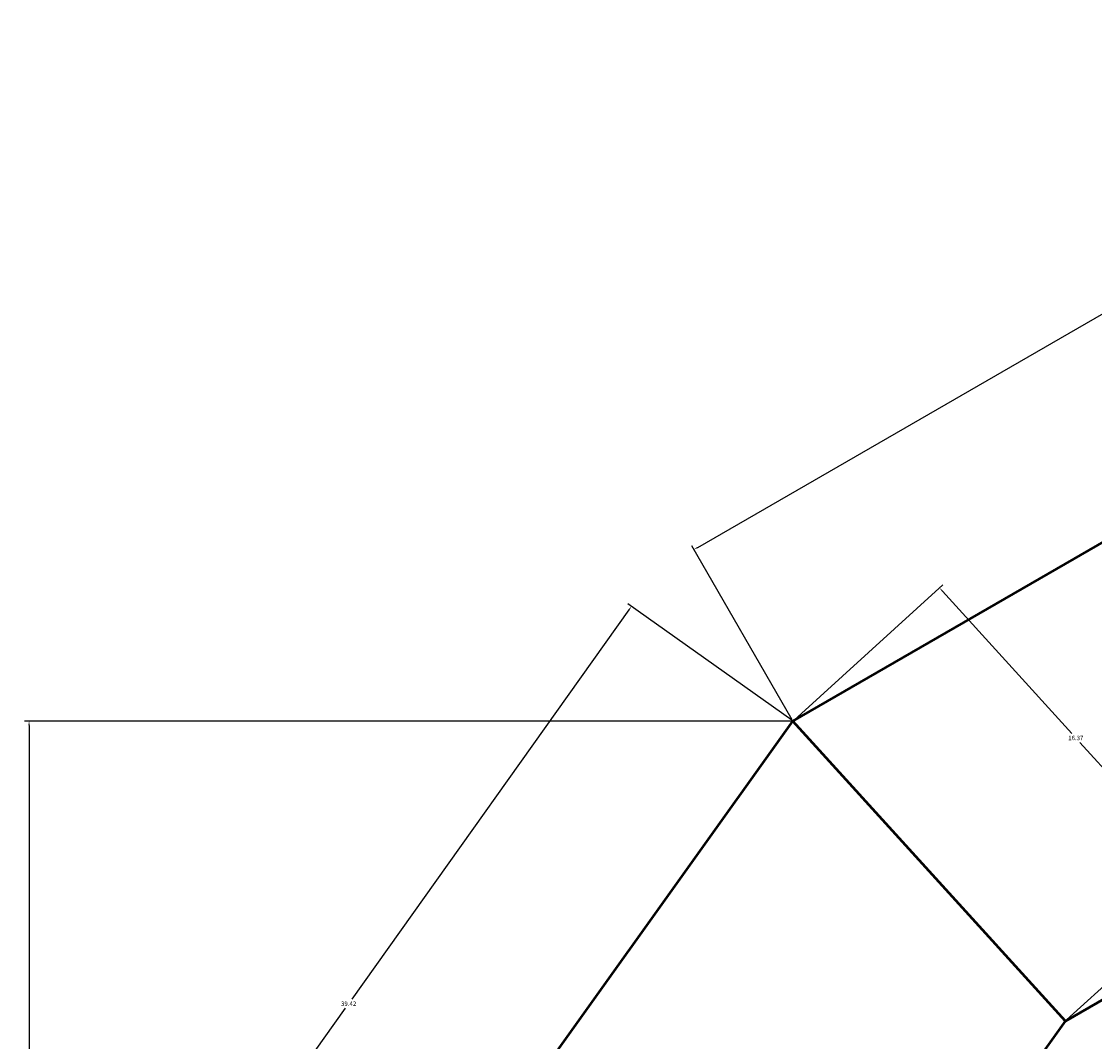
# Model space of a CAD drawing. Units: millimetres. Extents: x 2919 to 3075, y 2801 to 2951.
# Tile 7 of 14: x 2919 to 2963, y 2910 to 2951. Entities that reach past the tile are written whole.
import ezdxf

# ---------------------------------------------------------------- set-up
doc = ezdxf.new("R2010")
doc.units = ezdxf.units.MM
doc.layers.add('M-DIMS', color=2, linetype='Continuous', lineweight=18)
doc.layers.add('M-OUTL', color=7, linetype='Continuous', lineweight=50)
doc.styles.get("Standard").update_dxf_attribs({"font": 'arial.ttf'})
doc.dimstyles.get("Standard").update_dxf_attribs({"dimtxt": 0.18, "dimasz": 0.18, "dimexe": 0.18, "dimexo": 0.0625, "dimgap": 0.09, "dimtad": 0, "dimtih": 1, "dimtoh": 1, "dimdec": 4, "dimzin": 0, "dimdsep": 46, "dimtxsty": 'Standard', "dimcen": 0.09, "dimadec": 0, "dimazin": 0, "dimtfac": 1, "dimtdec": 4, "dimtofl": 0, "dimtmove": 0, "dimatfit": 3, "dimfxl": 1, "dimtolj": 1, "dimtzin": 0, "dimarcsym": 0})

# ---------------------------------------------------------------- blocks, each defined once
blk = doc.blocks.new('*D16')
at = {"layer": 'Defpoints', "color": 0, "transparency": 16777216}
for p in [(2983.323, 2951.131), (2987.323, 2944.203), (2950.626, 2923.015)]:
    blk.add_point(p, dxfattribs=at)
at = {"layer": 'M-DIMS', "color": 0, "lineweight": -2, "transparency": 16777216}
for p, q in [((2987.292, 2944.257), (2983.233, 2951.287)), ((2983.167, 2951.041), (2965.29, 2940.719)), ((2946.782, 2930.034), (2964.659, 2940.355)), ((2950.595, 2923.07), (2946.536, 2930.1))]:
    blk.add_line(p, q, dxfattribs=at)
at = {"layer": 'M-DIMS', "color": 0, "transparency": 16777216}
for points in [[(2983.152, 2951.067), (2983.182, 2951.015), (2983.323, 2951.131)], [(2946.767, 2930.06), (2946.797, 2930.008), (2946.626, 2929.944)]]:
    blk.add_solid(points, dxfattribs=at)
at = {"layer": 'M-DIMS', "color": 0, "transparency": 16777216, "insert": (2964.975, 2940.537), "char_height": 0.18, "attachment_point": 5}
blk.add_mtext('\\A1;42.374', dxfattribs=at)
blk = doc.blocks.new('*D21')
at = {"layer": 'Defpoints', "color": 0, "transparency": 16777216}
for p in [(2944.107, 2927.653), (2950.626, 2923.015), (2927.773, 2890.893)]:
    blk.add_point(p, dxfattribs=at)
at = {"layer": 'M-DIMS', "color": 0, "lineweight": -2, "transparency": 16777216}
for p, q in [((2950.575, 2923.052), (2943.961, 2927.757)), ((2944.003, 2927.506), (2932.81, 2911.774)), ((2921.359, 2895.677), (2932.551, 2911.41)), ((2927.722, 2890.929), (2921.108, 2895.635))]:
    blk.add_line(p, q, dxfattribs=at)
at = {"layer": 'M-DIMS', "color": 0, "transparency": 16777216}
for points in [[(2943.978, 2927.524), (2944.027, 2927.489), (2944.107, 2927.653)], [(2921.334, 2895.695), (2921.383, 2895.66), (2921.255, 2895.531)]]:
    blk.add_solid(points, dxfattribs=at)
at = {"layer": 'M-DIMS', "color": 0, "transparency": 16777216, "insert": (2932.681, 2911.592), "char_height": 0.18, "attachment_point": 5}
blk.add_mtext('\\A1;39.42', dxfattribs=at)
blk = doc.blocks.new('*D22')
at = {"layer": 'Defpoints', "color": 0, "transparency": 16777216}
for p in [(2950.626, 2923.015), (2967.553, 2916.27), (2961.63, 2910.893)]:
    blk.add_point(p, dxfattribs=at)
at = {"layer": 'M-DIMS', "color": 0, "lineweight": -2, "transparency": 16777216}
for p, q in [((2950.672, 2923.057), (2956.683, 2928.513)), ((2956.67, 2928.259), (2961.886, 2922.513)), ((2967.432, 2916.404), (2962.216, 2922.149)), ((2961.676, 2910.935), (2967.686, 2916.391))]:
    blk.add_line(p, q, dxfattribs=at)
at = {"layer": 'M-DIMS', "color": 0, "transparency": 16777216}
for points in [[(2956.693, 2928.279), (2956.648, 2928.239), (2956.549, 2928.392)], [(2967.454, 2916.424), (2967.41, 2916.383), (2967.553, 2916.27)]]:
    blk.add_solid(points, dxfattribs=at)
at = {"layer": 'M-DIMS', "color": 0, "transparency": 16777216, "insert": (2962.051, 2922.331), "char_height": 0.18, "attachment_point": 5}
blk.add_mtext('\\A1;16.37', dxfattribs=at)
blk = doc.blocks.new('*D23')
at = {"layer": 'Defpoints', "color": 0, "transparency": 16777216}
for p in [(2919.773, 2923.015), (2950.626, 2923.015), (2927.773, 2890.893)]:
    blk.add_point(p, dxfattribs=at)
at = {"layer": 'M-DIMS', "color": 0, "lineweight": -2, "transparency": 16777216}
for p, q in [((2950.563, 2923.015), (2919.593, 2923.015)), ((2919.773, 2922.835), (2919.773, 2907.136)), ((2919.773, 2891.073), (2919.773, 2906.772)), ((2927.711, 2890.893), (2919.593, 2890.893))]:
    blk.add_line(p, q, dxfattribs=at)
at = {"layer": 'M-DIMS', "color": 0, "transparency": 16777216}
for points in [[(2919.743, 2922.835), (2919.803, 2922.835), (2919.773, 2923.015)], [(2919.743, 2891.073), (2919.803, 2891.073), (2919.773, 2890.893)]]:
    blk.add_solid(points, dxfattribs=at)
at = {"layer": 'M-DIMS', "color": 0, "transparency": 16777216, "insert": (2919.773, 2906.954), "char_height": 0.18, "attachment_point": 5}
blk.add_mtext('\\A1;32.12', dxfattribs=at)

msp = doc.modelspace()

# ---------------------------------------------------------------- linework, layer by layer
at = {"layer": 'M-OUTL'}
msp.add_line((2961.6296, 2910.8932), (2950.6258, 2923.0154), dxfattribs=at)
for points in [[(2928.6099, 2892.1931), (2950.6258, 2923.0154), (2987.3232, 2944.2026)], [(2941.6296, 2882.8932), (2961.6296, 2910.8932), (2995.3232, 2930.3462)], [(2941.6296, 2882.8932), (2961.6296, 2910.8932), (2995.3232, 2930.3462)]]:
    msp.add_lwpolyline(points, dxfattribs=at)

# ---------------------------------------------------------------- dimensions: what is measured, and where the dimension line sits
at = {"layer": 'M-DIMS'}
for base, p1, p2, angle, override, picture, middle in [((2983.3232, 2951.1308), (2950.6258, 2923.0154), (2987.3232, 2944.2026), 30, {"dimdec": 3, "dimlfac": 1, "dimrnd": 0, "dimzin": 0, "dimdsep": 46, "dimlunit": 2}, '*D16', (2964.9745, 2940.5372)), ((2967.5531, 2916.2702), (2950.6258, 2923.0154), (2961.6296, 2910.8932), 312.23116, {"dimdec": 2, "dimlfac": 1, "dimrnd": 0, "dimzin": 0, "dimdsep": 46, "dimlunit": 2}, '*D22', (2962.0512, 2922.3313)), ((2944.1072, 2927.653), (2927.7732, 2890.8932), (2950.6258, 2923.0154), 54.57085, {"dimdec": 2, "dimlfac": 1, "dimrnd": 0, "dimzin": 0, "dimdsep": 46, "dimlunit": 2}, '*D21', (2932.6808, 2911.5919)), ((2919.7732, 2923.0154), (2927.7732, 2890.8932), (2950.6258, 2923.0154), 90, {"dimdec": 2, "dimlfac": 1, "dimrnd": 0, "dimzin": 0, "dimdsep": 46, "dimlunit": 2}, '*D23', (2919.7732, 2906.9543))]:
    dim = msp.add_linear_dim(base=base, p1=p1, p2=p2, angle=angle, dimstyle='Standard', override=override, dxfattribs=at)
    dim.commit()
    dim.dimension.update_dxf_attribs({"geometry": picture, "text_midpoint": middle})

doc.saveas('drawing.dxf')
